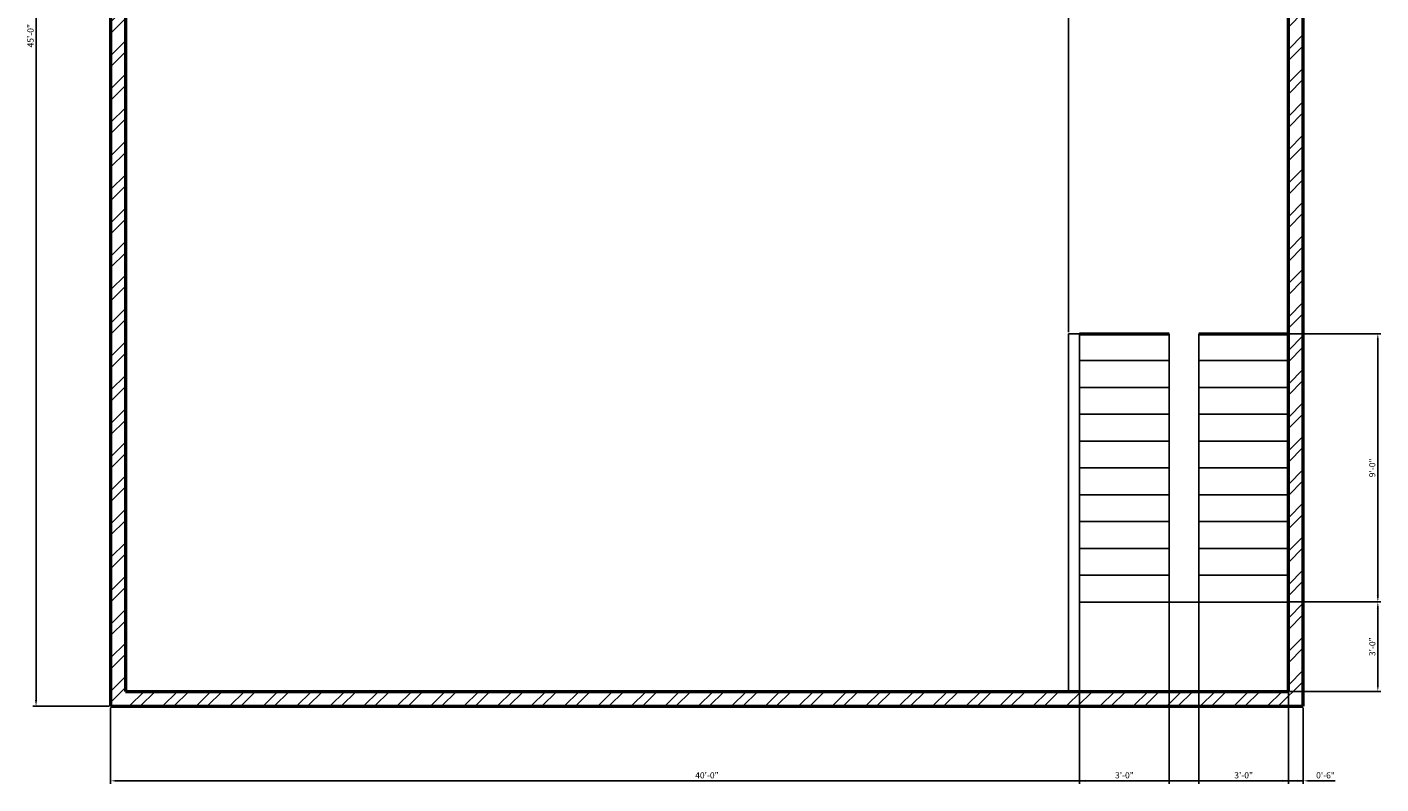
# Model space of a CAD drawing. Units: inches. Extents: x 244 to 2800, y 1060 to 1700.
# Tile 1 of 13: x 244 to 789, y 1062 to 1366. Entities that reach past the tile are written whole.
import ezdxf

# ---------------------------------------------------------------- set-up
doc = ezdxf.new("R2010")
doc.units = ezdxf.units.IN
for name, color, linetype, lineweight in [('A-ANNO-DIMS', 2, 'Continuous', 18), ('A-FLOR-STRS', 6, 'Continuous', 25), ('A-WALL', 7, 'Continuous', 50), ('A-WALL-PATT', 8, 'Continuous', 13)]:
    doc.layers.add(name, color=color, linetype=linetype, lineweight=lineweight)
doc.styles.get("Standard").update_dxf_attribs({"font": 'arial.ttf'})
doc.dimstyles.new('ISO-25', dxfattribs={"dimtxt": 2.5, "dimasz": 2.5, "dimexe": 1.25, "dimexo": 0.625, "dimtad": 1, "dimlunit": 4, "dimtxsty": 'Standard', "dimcen": 2.5, "dimadec": 0, "dimazin": 0, "dimtfac": 1, "dimtmove": 0, "dimatfit": 3, "dimfxl": 1, "dimarcsym": 0})

# ---------------------------------------------------------------- blocks, each defined once
blk = doc.blocks.new('*D156')
at = {"layer": 'A-ANNO-DIMS', "color": 0, "lineweight": -2, "transparency": 16777216}
for p, q in [((277.3, 1092.36), (277.3, 1061.74)), ((757.3, 1092.36), (757.3, 1061.74)), ((279.8, 1062.99), (754.8, 1062.99))]:
    blk.add_line(p, q, dxfattribs=at)
at = {"layer": 'A-ANNO-DIMS', "color": 0, "transparency": 16777216}
for points in [[(279.8, 1063.4), (279.8, 1062.57), (277.3, 1062.99)], [(754.8, 1063.4), (754.8, 1062.57), (757.3, 1062.99)]]:
    blk.add_solid(points, dxfattribs=at)
at = {"layer": 'Defpoints', "color": 0, "transparency": 16777216}
for p in [(277.3, 1092.99), (757.3, 1092.99), (757.3, 1062.99)]:
    blk.add_point(p, dxfattribs=at)
at = {"layer": 'A-ANNO-DIMS', "color": 0, "transparency": 16777216, "insert": (517.3, 1064.89), "char_height": 2.5, "attachment_point": 5}
blk.add_mtext('40\'-0"', dxfattribs=at)
blk = doc.blocks.new('*D157')
at = {"layer": 'A-ANNO-DIMS', "color": 0, "lineweight": -2, "transparency": 16777216}
for p, q in [((276.67, 1632.99), (246.05, 1632.99)), ((247.3, 1095.49), (247.3, 1630.49)), ((276.67, 1092.99), (246.05, 1092.99))]:
    blk.add_line(p, q, dxfattribs=at)
at = {"layer": 'A-ANNO-DIMS', "color": 0, "transparency": 16777216}
for points in [[(246.88, 1630.49), (247.71, 1630.49), (247.3, 1632.99)], [(246.88, 1095.49), (247.71, 1095.49), (247.3, 1092.99)]]:
    blk.add_solid(points, dxfattribs=at)
at = {"layer": 'Defpoints', "color": 0, "transparency": 16777216}
for p in [(247.3, 1632.99), (277.3, 1632.99), (277.3, 1092.99)]:
    blk.add_point(p, dxfattribs=at)
at = {"layer": 'A-ANNO-DIMS', "color": 0, "transparency": 16777216, "insert": (245.39, 1362.99), "char_height": 2.5, "attachment_point": 5, "rotation": 90}
blk.add_mtext('45\'-0"', dxfattribs=at)
blk = doc.blocks.new('*D158')
at = {"layer": 'A-ANNO-DIMS', "color": 0, "lineweight": -2, "transparency": 16777216}
for p, q in [((662.8, 1243.61), (662.8, 1664.24)), ((665.3, 1662.99), (748.8, 1662.99)), ((751.3, 1243.61), (751.3, 1664.24))]:
    blk.add_line(p, q, dxfattribs=at)
at = {"layer": 'A-ANNO-DIMS', "color": 0, "transparency": 16777216}
for points in [[(665.3, 1663.4), (665.3, 1662.57), (662.8, 1662.99)], [(748.8, 1663.4), (748.8, 1662.57), (751.3, 1662.99)]]:
    blk.add_solid(points, dxfattribs=at)
at = {"layer": 'Defpoints', "color": 0, "transparency": 16777216}
for p in [(751.3, 1662.99), (662.8, 1242.99), (751.3, 1242.99)]:
    blk.add_point(p, dxfattribs=at)
at = {"layer": 'A-ANNO-DIMS', "color": 0, "transparency": 16777216, "insert": (707.05, 1664.9), "char_height": 2.5, "attachment_point": 5}
blk.add_mtext('7\'-4 1/2"', dxfattribs=at)
blk = doc.blocks.new('*D159')
at = {"layer": 'A-ANNO-DIMS', "color": 0, "lineweight": -2, "transparency": 16777216}
for p, q in [((751.92, 1134.99), (788.55, 1134.99)), ((787.3, 1101.49), (787.3, 1132.49)), ((751.92, 1098.99), (788.55, 1098.99))]:
    blk.add_line(p, q, dxfattribs=at)
at = {"layer": 'A-ANNO-DIMS', "color": 0, "transparency": 16777216}
for points in [[(786.88, 1132.49), (787.71, 1132.49), (787.3, 1134.99)], [(786.88, 1101.49), (787.71, 1101.49), (787.3, 1098.99)]]:
    blk.add_solid(points, dxfattribs=at)
at = {"layer": 'Defpoints', "color": 0, "transparency": 16777216}
for p in [(751.3, 1134.99), (787.3, 1134.99), (751.3, 1098.99)]:
    blk.add_point(p, dxfattribs=at)
at = {"layer": 'A-ANNO-DIMS', "color": 0, "transparency": 16777216, "insert": (785.39, 1116.99), "char_height": 2.5, "attachment_point": 5, "rotation": 90}
blk.add_mtext('3\'-0"', dxfattribs=at)
blk = doc.blocks.new('*D160')
at = {"layer": 'A-ANNO-DIMS', "color": 0, "lineweight": -2, "transparency": 16777216}
for p, q in [((751.92, 1242.99), (788.55, 1242.99)), ((787.3, 1137.49), (787.3, 1240.49)), ((751.92, 1134.99), (788.55, 1134.99))]:
    blk.add_line(p, q, dxfattribs=at)
at = {"layer": 'A-ANNO-DIMS', "color": 0, "transparency": 16777216}
for points in [[(786.88, 1240.49), (787.71, 1240.49), (787.3, 1242.99)], [(786.88, 1137.49), (787.71, 1137.49), (787.3, 1134.99)]]:
    blk.add_solid(points, dxfattribs=at)
at = {"layer": 'Defpoints', "color": 0, "transparency": 16777216}
for p in [(751.3, 1242.99), (787.3, 1242.99), (751.3, 1134.99)]:
    blk.add_point(p, dxfattribs=at)
at = {"layer": 'A-ANNO-DIMS', "color": 0, "transparency": 16777216, "insert": (785.39, 1188.99), "char_height": 2.5, "attachment_point": 5, "rotation": 90}
blk.add_mtext('9\'-0"', dxfattribs=at)
blk = doc.blocks.new('*D161')
at = {"layer": 'A-ANNO-DIMS', "color": 0, "lineweight": -2, "transparency": 16777216}
for p, q in [((667.3, 1242.36), (667.3, 1061.74)), ((703.3, 1242.36), (703.3, 1061.74)), ((669.8, 1062.99), (700.8, 1062.99))]:
    blk.add_line(p, q, dxfattribs=at)
at = {"layer": 'A-ANNO-DIMS', "color": 0, "transparency": 16777216}
for points in [[(669.8, 1063.4), (669.8, 1062.57), (667.3, 1062.99)], [(700.8, 1063.4), (700.8, 1062.57), (703.3, 1062.99)]]:
    blk.add_solid(points, dxfattribs=at)
at = {"layer": 'Defpoints', "color": 0, "transparency": 16777216}
for p in [(667.3, 1242.99), (703.3, 1242.99), (703.3, 1062.99)]:
    blk.add_point(p, dxfattribs=at)
at = {"layer": 'A-ANNO-DIMS', "color": 0, "transparency": 16777216, "insert": (685.3, 1064.89), "char_height": 2.5, "attachment_point": 5}
blk.add_mtext('3\'-0"', dxfattribs=at)
blk = doc.blocks.new('*D162')
at = {"layer": 'A-ANNO-DIMS', "color": 0, "lineweight": -2, "transparency": 16777216}
for p, q in [((715.3, 1242.36), (715.3, 1061.74)), ((751.3, 1242.36), (751.3, 1061.74)), ((717.8, 1062.99), (748.8, 1062.99))]:
    blk.add_line(p, q, dxfattribs=at)
at = {"layer": 'A-ANNO-DIMS', "color": 0, "transparency": 16777216}
for points in [[(717.8, 1063.4), (717.8, 1062.57), (715.3, 1062.99)], [(748.8, 1063.4), (748.8, 1062.57), (751.3, 1062.99)]]:
    blk.add_solid(points, dxfattribs=at)
at = {"layer": 'Defpoints', "color": 0, "transparency": 16777216}
for p in [(715.3, 1242.99), (751.3, 1242.99), (751.3, 1062.99)]:
    blk.add_point(p, dxfattribs=at)
at = {"layer": 'A-ANNO-DIMS', "color": 0, "transparency": 16777216, "insert": (733.3, 1064.89), "char_height": 2.5, "attachment_point": 5}
blk.add_mtext('3\'-0"', dxfattribs=at)
blk = doc.blocks.new('*D163')
at = {"layer": 'A-ANNO-DIMS', "color": 0, "lineweight": -2, "transparency": 16777216}
for p, q in [((751.3, 1098.36), (751.3, 1061.74)), ((757.3, 1092.36), (757.3, 1061.74)), ((748.8, 1062.99), (746.3, 1062.99)), ((751.3, 1062.99), (757.3, 1062.99)), ((759.8, 1062.99), (770.19, 1062.99))]:
    blk.add_line(p, q, dxfattribs=at)
at = {"layer": 'A-ANNO-DIMS', "color": 0, "transparency": 16777216}
for points in [[(748.8, 1063.4), (748.8, 1062.57), (751.3, 1062.99)], [(759.8, 1063.4), (759.8, 1062.57), (757.3, 1062.99)]]:
    blk.add_solid(points, dxfattribs=at)
at = {"layer": 'Defpoints', "color": 0, "transparency": 16777216}
for p in [(751.3, 1098.99), (757.3, 1092.99), (757.3, 1062.99)]:
    blk.add_point(p, dxfattribs=at)
at = {"layer": 'A-ANNO-DIMS', "color": 0, "transparency": 16777216, "insert": (766.24, 1064.89), "char_height": 2.5, "attachment_point": 5}
blk.add_mtext('0\'-6"', dxfattribs=at)

msp = doc.modelspace()

# ---------------------------------------------------------------- hatches: boundary and pattern name
at = {"layer": 'A-WALL-PATT'}
h = msp.add_hatch(dxfattribs=at)
h.set_pattern_fill('ANSI32', color=256)
h.paths.add_polyline_path([(757.295, 1632.986), (277.295, 1632.986), (277.295, 1092.986), (757.295, 1092.986)])
h.paths.add_polyline_path([(283.295, 1098.986), (283.295, 1626.986), (751.295, 1626.986), (751.295, 1098.986), (667.295, 1098.986)], flags=16)
h.paths.add_polyline_path([(667.295, 1242.986), (703.295, 1242.986), (703.295, 1134.986), (715.295, 1134.986), (715.295, 1242.986), (751.295, 1242.986), (751.295, 1134.986), (667.295, 1134.986)], flags=0)

# ---------------------------------------------------------------- linework, layer by layer
at = {"layer": 'A-FLOR-STRS'}
for p, q in [((662.795, 1098.986), (662.795, 1242.986)), ((662.795, 1242.986), (667.295, 1242.986)), ((667.295, 1242.986), (703.295, 1242.986)), ((667.295, 1242.986), (667.295, 1098.986)), ((667.295, 1242.986), (703.295, 1242.986)), ((667.295, 1098.986), (667.295, 1242.986)), ((703.295, 1242.986), (703.295, 1134.986)), ((715.295, 1242.986), (751.295, 1242.986)), ((715.295, 1242.986), (715.295, 1134.986)), ((715.295, 1242.986), (751.295, 1242.986)), ((751.295, 1242.986), (751.295, 1098.986)), ((667.295, 1232.186), (703.295, 1232.186)), ((715.295, 1232.186), (751.295, 1232.186)), ((667.295, 1221.386), (703.295, 1221.386)), ((715.295, 1221.386), (751.295, 1221.386)), ((667.295, 1210.586), (703.295, 1210.586)), ((715.295, 1210.586), (751.295, 1210.586)), ((667.295, 1199.786), (703.295, 1199.786)), ((715.295, 1199.786), (751.295, 1199.786)), ((667.295, 1188.986), (703.295, 1188.986)), ((715.295, 1188.986), (751.295, 1188.986)), ((667.295, 1178.186), (703.295, 1178.186)), ((715.295, 1178.186), (751.295, 1178.186)), ((667.295, 1167.386), (703.295, 1167.386)), ((715.295, 1167.386), (751.295, 1167.386)), ((667.295, 1156.586), (703.295, 1156.586)), ((715.295, 1156.586), (751.295, 1156.586)), ((667.295, 1145.786), (703.295, 1145.786)), ((715.295, 1145.786), (751.295, 1145.786)), ((667.295, 1134.986), (751.295, 1134.986)), ((667.295, 1098.986), (751.295, 1098.986))]:
    msp.add_line(p, q, dxfattribs=at)
at = {"layer": 'A-WALL'}
for p, q in [((277.295, 1632.986), (277.295, 1092.986)), ((757.295, 1092.986), (757.295, 1632.986)), ((283.295, 1626.986), (283.295, 1098.986)), ((751.295, 1098.986), (751.295, 1626.986)), ((667.295, 1242.986), (703.295, 1242.986)), ((715.295, 1242.986), (751.295, 1242.986)), ((283.295, 1098.986), (751.295, 1098.986)), ((277.295, 1092.986), (757.295, 1092.986))]:
    msp.add_line(p, q, dxfattribs=at)

# ---------------------------------------------------------------- dimensions: what is measured, and where the dimension line sits
at = {"layer": 'A-ANNO-DIMS'}
for base, p1, p2, picture, middle in [((751.295, 1662.986), (662.795, 1242.986), (751.295, 1242.986), '*D158', (707.045, 1664.904)), ((703.295, 1062.986), (667.295, 1242.986), (703.295, 1242.986), '*D161', (685.295, 1064.888)), ((751.295, 1062.986), (715.295, 1242.986), (751.295, 1242.986), '*D162', (733.295, 1064.888)), ((757.295, 1062.986), (751.295, 1098.986), (757.295, 1092.986), '*D163', (766.243, 1064.888)), ((757.295, 1062.986), (277.295, 1092.986), (757.295, 1092.986), '*D156', (517.295, 1064.888))]:
    dim = msp.add_linear_dim(base=base, p1=p1, p2=p2, dimstyle='ISO-25', override={"dimdec": 1, "dimlfac": 1, "dimrnd": 0, "dimzin": 1, "dimdsep": 46, "dimlunit": 4, "dimfrac": 2}, dxfattribs=at)
    dim.commit()
    dim.dimension.update_dxf_attribs({"geometry": picture, "text_midpoint": middle})
for base, p1, p2, picture, middle in [((247.295, 1632.986), (277.295, 1092.986), (277.295, 1632.986), '*D157', (245.394, 1362.986)), ((787.295, 1242.986), (751.295, 1134.986), (751.295, 1242.986), '*D160', (785.394, 1188.986)), ((787.295, 1134.986), (751.295, 1098.986), (751.295, 1134.986), '*D159', (785.393, 1116.986))]:
    dim = msp.add_linear_dim(base=base, p1=p1, p2=p2, angle=90, dimstyle='ISO-25', override={"dimdec": 1, "dimlfac": 1, "dimrnd": 0, "dimzin": 1, "dimdsep": 46, "dimlunit": 4, "dimfrac": 2}, dxfattribs=at)
    dim.commit()
    dim.dimension.update_dxf_attribs({"geometry": picture, "text_midpoint": middle})

doc.saveas('drawing.dxf')
